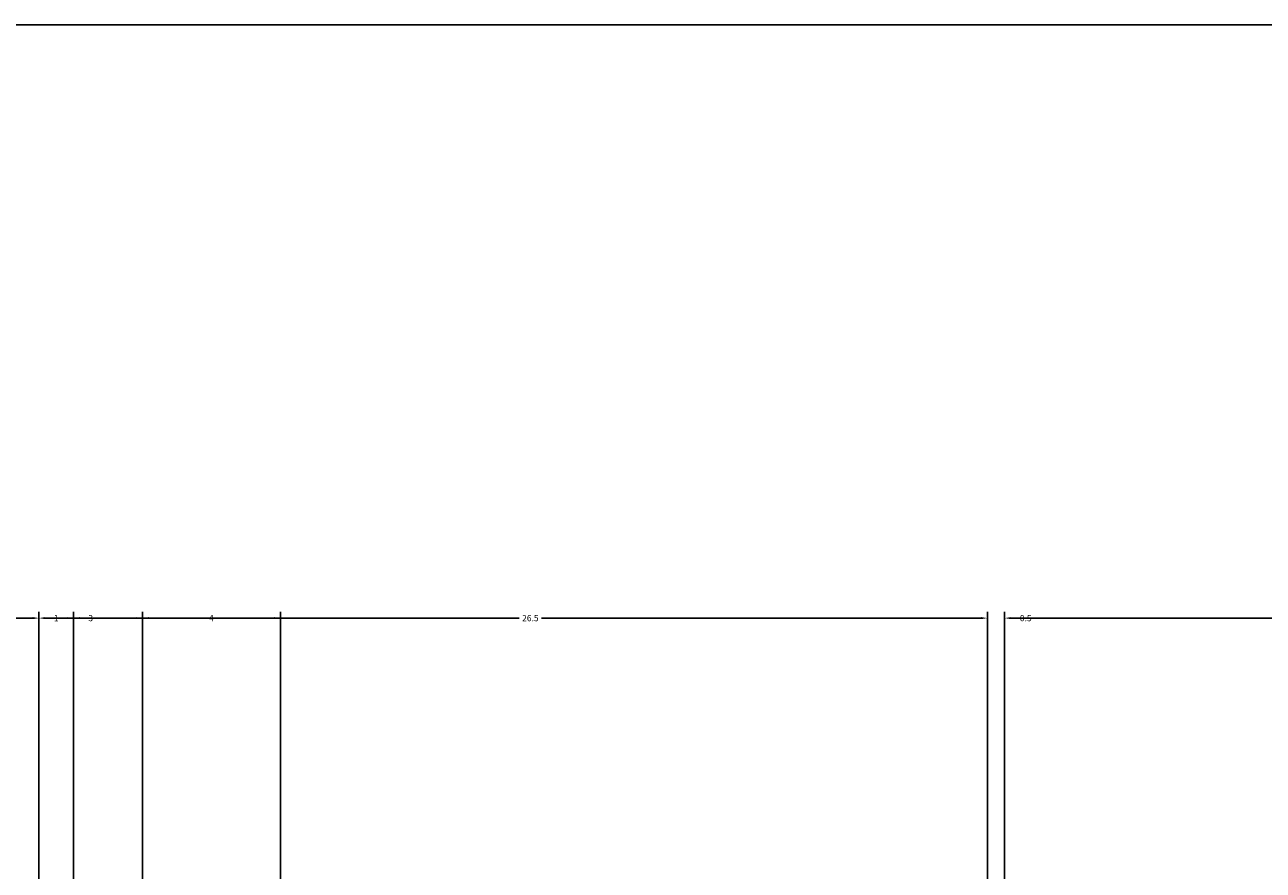
# Model space of a CAD drawing. Units: inches. Extents: x 4508 to 4723, y 847 to 1020.
# Tile 16 of 32: x 4550 to 4585, y 995 to 1020. Entities that reach past the tile are written whole.
import ezdxf

# ---------------------------------------------------------------- set-up
doc = ezdxf.new("R2010")
doc.units = ezdxf.units.IN
doc.layers.add('A-ANNO-DIMS', color=2, linetype='Continuous', lineweight=18)
doc.layers.add('A-ANNO-TTLB', color=7, linetype='Continuous', lineweight=25)
doc.styles.get("Standard").update_dxf_attribs({"font": 'arial.ttf'})
doc.dimstyles.get("Standard").update_dxf_attribs({"dimtxt": 0.18, "dimasz": 0.18, "dimexe": 0.18, "dimexo": 0.0625, "dimgap": 0.09, "dimtad": 0, "dimtih": 1, "dimtoh": 1, "dimdec": 4, "dimzin": 0, "dimdsep": 46, "dimtxsty": 'Standard', "dimcen": 0.09, "dimadec": 0, "dimazin": 0, "dimtfac": 1, "dimtdec": 4, "dimtofl": 0, "dimtmove": 0, "dimatfit": 3, "dimfxl": 1, "dimtolj": 1, "dimtzin": 0, "dimarcsym": 0})

# ---------------------------------------------------------------- blocks, each defined once
blk = doc.blocks.new('*D4')
at = {"layer": 'A-ANNO-DIMS', "color": 0, "lineweight": -2, "transparency": 16777216}
for p, q in [((4540.994, 994.809), (4540.994, 1002.877)), ((4541.174, 1002.697), (4545.345, 1002.697)), ((4549.814, 1002.697), (4545.643, 1002.697)), ((4549.994, 994.809), (4549.994, 1002.877))]:
    blk.add_line(p, q, dxfattribs=at)
at = {"layer": 'A-ANNO-DIMS', "color": 0, "lineweight": 9, "transparency": 16777216}
for points in [[(4541.174, 1002.727), (4541.174, 1002.667), (4540.994, 1002.697)], [(4549.814, 1002.727), (4549.814, 1002.667), (4549.994, 1002.697)]]:
    blk.add_solid(points, dxfattribs=at)
at = {"layer": 'Defpoints', "color": 0, "lineweight": 9, "transparency": 16777216}
for p in [(4549.994, 1002.697), (4540.994, 994.747), (4549.994, 994.747)]:
    blk.add_point(p, dxfattribs=at)
at = {"layer": 'A-ANNO-DIMS', "color": 0, "transparency": 16777216, "insert": (4545.494, 1002.697), "char_height": 0.18, "attachment_point": 5}
blk.add_mtext('\\A1;9', dxfattribs=at)
blk = doc.blocks.new('*D5')
at = {"layer": 'A-ANNO-DIMS', "color": 0, "lineweight": -2, "transparency": 16777216}
for p, q in [((4549.994, 994.809), (4549.994, 1002.877)), ((4550.174, 1002.697), (4551.345, 1002.697)), ((4552.814, 1002.697), (4551.643, 1002.697)), ((4552.994, 994.809), (4552.994, 1002.877))]:
    blk.add_line(p, q, dxfattribs=at)
at = {"layer": 'A-ANNO-DIMS', "color": 0, "lineweight": 9, "transparency": 16777216}
for points in [[(4550.174, 1002.727), (4550.174, 1002.667), (4549.994, 1002.697)], [(4552.814, 1002.727), (4552.814, 1002.667), (4552.994, 1002.697)]]:
    blk.add_solid(points, dxfattribs=at)
at = {"layer": 'Defpoints', "color": 0, "lineweight": 9, "transparency": 16777216}
for p in [(4552.994, 1002.697), (4549.994, 994.747), (4552.994, 994.747)]:
    blk.add_point(p, dxfattribs=at)
at = {"layer": 'A-ANNO-DIMS', "color": 0, "transparency": 16777216, "insert": (4551.494, 1002.697), "char_height": 0.18, "attachment_point": 5}
blk.add_mtext('\\A1;3', dxfattribs=at)
blk = doc.blocks.new('*D6')
at = {"layer": 'A-ANNO-DIMS', "color": 0, "lineweight": -2, "transparency": 16777216}
for p, q in [((4552.994, 994.809), (4552.994, 1002.877)), ((4553.174, 1002.697), (4554.842, 1002.697)), ((4556.814, 1002.697), (4555.146, 1002.697)), ((4556.994, 994.809), (4556.994, 1002.877))]:
    blk.add_line(p, q, dxfattribs=at)
at = {"layer": 'A-ANNO-DIMS', "color": 0, "lineweight": 9, "transparency": 16777216}
for points in [[(4553.174, 1002.727), (4553.174, 1002.667), (4552.994, 1002.697)], [(4556.814, 1002.727), (4556.814, 1002.667), (4556.994, 1002.697)]]:
    blk.add_solid(points, dxfattribs=at)
at = {"layer": 'Defpoints', "color": 0, "lineweight": 9, "transparency": 16777216}
for p in [(4556.994, 1002.697), (4552.994, 994.747), (4556.994, 994.747)]:
    blk.add_point(p, dxfattribs=at)
at = {"layer": 'A-ANNO-DIMS', "color": 0, "transparency": 16777216, "insert": (4554.994, 1002.697), "char_height": 0.18, "attachment_point": 5}
blk.add_mtext('\\A1;4', dxfattribs=at)
blk = doc.blocks.new('*D26')
at = {"layer": 'A-ANNO-DIMS', "color": 0, "lineweight": -2, "transparency": 16777216}
for p, q in [((4549.994, 904.809), (4549.994, 1002.877)), ((4550.174, 1002.697), (4550.371, 1002.697)), ((4550.814, 1002.697), (4550.617, 1002.697)), ((4550.994, 903.809), (4550.994, 1002.877))]:
    blk.add_line(p, q, dxfattribs=at)
at = {"layer": 'A-ANNO-DIMS', "color": 0, "lineweight": 9, "transparency": 16777216}
for points in [[(4550.174, 1002.727), (4550.174, 1002.667), (4549.994, 1002.697)], [(4550.814, 1002.727), (4550.814, 1002.667), (4550.994, 1002.697)]]:
    blk.add_solid(points, dxfattribs=at)
at = {"layer": 'Defpoints', "color": 0, "lineweight": 9, "transparency": 16777216}
for p in [(4550.994, 1002.697), (4549.994, 904.747), (4550.994, 903.747)]:
    blk.add_point(p, dxfattribs=at)
at = {"layer": 'A-ANNO-DIMS', "color": 0, "transparency": 16777216, "insert": (4550.494, 1002.697), "char_height": 0.18, "attachment_point": 5}
blk.add_mtext('\\A1;1', dxfattribs=at)
blk = doc.blocks.new('*D27')
at = {"layer": 'A-ANNO-DIMS', "color": 0, "lineweight": -2, "transparency": 16777216}
for p, q in [((4550.994, 903.809), (4550.994, 1002.877)), ((4551.174, 1002.697), (4563.918, 1002.697)), ((4577.314, 1002.697), (4564.57, 1002.697)), ((4577.494, 903.809), (4577.494, 1002.877))]:
    blk.add_line(p, q, dxfattribs=at)
at = {"layer": 'A-ANNO-DIMS', "color": 0, "lineweight": 9, "transparency": 16777216}
for points in [[(4551.174, 1002.727), (4551.174, 1002.667), (4550.994, 1002.697)], [(4577.314, 1002.727), (4577.314, 1002.667), (4577.494, 1002.697)]]:
    blk.add_solid(points, dxfattribs=at)
at = {"layer": 'Defpoints', "color": 0, "lineweight": 9, "transparency": 16777216}
for p in [(4577.494, 1002.697), (4550.994, 903.747), (4577.494, 903.747)]:
    blk.add_point(p, dxfattribs=at)
at = {"layer": 'A-ANNO-DIMS', "color": 0, "transparency": 16777216, "insert": (4564.244, 1002.697), "char_height": 0.18, "attachment_point": 5}
blk.add_mtext('\\A1;26.5', dxfattribs=at)
blk = doc.blocks.new('*D28')
at = {"layer": 'A-ANNO-DIMS', "color": 0, "lineweight": -2, "transparency": 16777216}
for p, q in [((4577.314, 1002.697), (4577.134, 1002.697)), ((4577.494, 903.809), (4577.494, 1002.877)), ((4577.994, 903.809), (4577.994, 1002.877)), ((4578.174, 1002.697), (4578.354, 1002.697))]:
    blk.add_line(p, q, dxfattribs=at)
at = {"layer": 'A-ANNO-DIMS', "color": 0, "lineweight": 9, "transparency": 16777216}
for points in [[(4577.314, 1002.727), (4577.314, 1002.667), (4577.494, 1002.697)], [(4578.174, 1002.727), (4578.174, 1002.667), (4577.994, 1002.697)]]:
    blk.add_solid(points, dxfattribs=at)
at = {"layer": 'Defpoints', "color": 0, "lineweight": 9, "transparency": 16777216}
for p in [(4577.994, 1002.697), (4577.494, 903.747), (4577.994, 903.747)]:
    blk.add_point(p, dxfattribs=at)
at = {"layer": 'A-ANNO-DIMS', "color": 0, "transparency": 16777216, "insert": (4578.608, 1002.697), "char_height": 0.18, "attachment_point": 5}
blk.add_mtext('\\A1;0.5', dxfattribs=at)
blk = doc.blocks.new('*D29')
at = {"layer": 'A-ANNO-DIMS', "color": 0, "lineweight": -2, "transparency": 16777216}
for p, q in [((4577.994, 903.809), (4577.994, 1002.877)), ((4578.174, 1002.697), (4590.773, 1002.697)), ((4603.814, 1002.697), (4591.214, 1002.697)), ((4603.994, 903.809), (4603.994, 1002.877))]:
    blk.add_line(p, q, dxfattribs=at)
at = {"layer": 'A-ANNO-DIMS', "color": 0, "lineweight": 9, "transparency": 16777216}
for points in [[(4578.174, 1002.727), (4578.174, 1002.667), (4577.994, 1002.697)], [(4603.814, 1002.727), (4603.814, 1002.667), (4603.994, 1002.697)]]:
    blk.add_solid(points, dxfattribs=at)
at = {"layer": 'Defpoints', "color": 0, "lineweight": 9, "transparency": 16777216}
for p in [(4603.994, 1002.697), (4577.994, 903.747), (4603.994, 903.747)]:
    blk.add_point(p, dxfattribs=at)
at = {"layer": 'A-ANNO-DIMS', "color": 0, "transparency": 16777216, "insert": (4590.994, 1002.697), "char_height": 0.18, "attachment_point": 5}
blk.add_mtext('\\A1;26', dxfattribs=at)

msp = doc.modelspace()

# ---------------------------------------------------------------- linework, layer by layer
at = {"layer": 'A-ANNO-TTLB'}
msp.add_lwpolyline([(4508.3867, 1019.9118), (4722.9774, 1019.9118), (4722.9774, 846.9535), (4508.3867, 846.9535)], close=True, dxfattribs=at)

# ---------------------------------------------------------------- dimensions: what is measured, and where the dimension line sits
at = {"layer": 'A-ANNO-DIMS'}
for base, p1, p2, override, picture, middle in [((4549.9938, 1002.6969), (4540.9938, 994.7469), (4549.9938, 994.7469), {"dimdec": 0, "dimlfac": 1, "dimrnd": 0, "dimzin": 0, "dimdsep": 46, "dimlunit": 2}, '*D4', (4545.4938, 1002.6969)), ((4552.9938, 1002.6969), (4549.9938, 994.7469), (4552.9938, 994.7469), {"dimdec": 0, "dimlfac": 1, "dimrnd": 0, "dimzin": 0, "dimdsep": 46, "dimlunit": 2}, '*D5', (4551.4938, 1002.6969)), ((4550.9938, 1002.6969), (4549.9938, 904.7469), (4550.9938, 903.7469), {"dimdec": 0, "dimlfac": 1, "dimrnd": 0, "dimzin": 0, "dimdsep": 46, "dimlunit": 2}, '*D26', (4550.4938, 1002.6969)), ((4577.4938, 1002.6969), (4550.9938, 903.7469), (4577.4938, 903.7469), {"dimdec": 1, "dimlfac": 1, "dimrnd": 0, "dimzin": 0, "dimdsep": 46, "dimlunit": 2}, '*D27', (4564.2438, 1002.6969)), ((4556.9938, 1002.6969), (4552.9938, 994.7469), (4556.9938, 994.7469), {"dimdec": 0, "dimlfac": 1, "dimrnd": 0, "dimzin": 0, "dimdsep": 46, "dimlunit": 2}, '*D6', (4554.9938, 1002.6969)), ((4577.9938, 1002.6969), (4577.4938, 903.7469), (4577.9938, 903.7469), {"dimdec": 1, "dimlfac": 1, "dimrnd": 0, "dimzin": 0, "dimdsep": 46, "dimlunit": 2}, '*D28', (4578.6083, 1002.6969)), ((4603.9938, 1002.6969), (4577.9938, 903.7469), (4603.9938, 903.7469), {"dimdec": 0, "dimlfac": 1, "dimrnd": 0, "dimzin": 0, "dimdsep": 46, "dimlunit": 2}, '*D29', (4590.9938, 1002.6969))]:
    dim = msp.add_linear_dim(base=base, p1=p1, p2=p2, dimstyle='Standard', override=override, dxfattribs=at)
    dim.commit()
    dim.dimension.update_dxf_attribs({"geometry": picture, "text_midpoint": middle})

doc.saveas('drawing.dxf')
